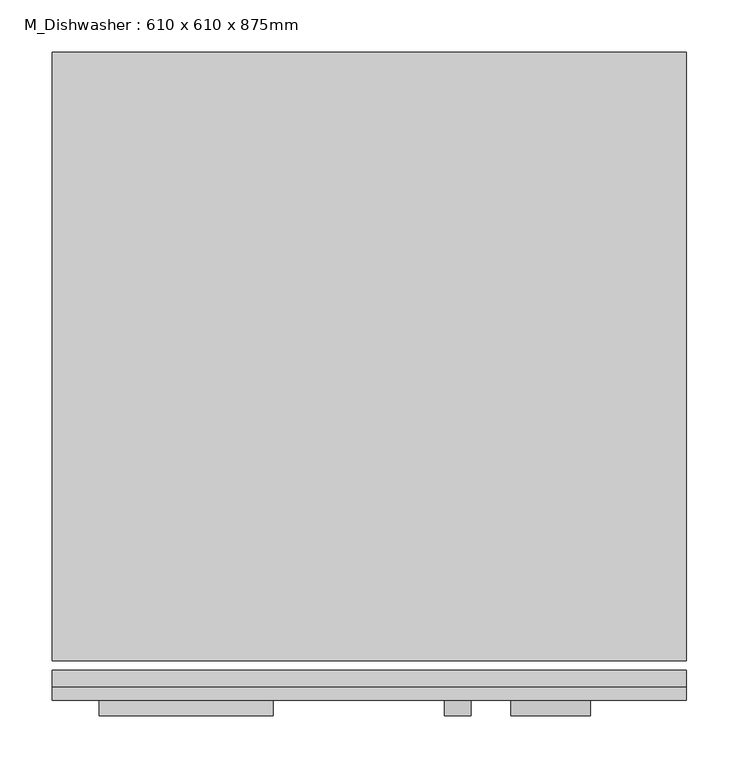
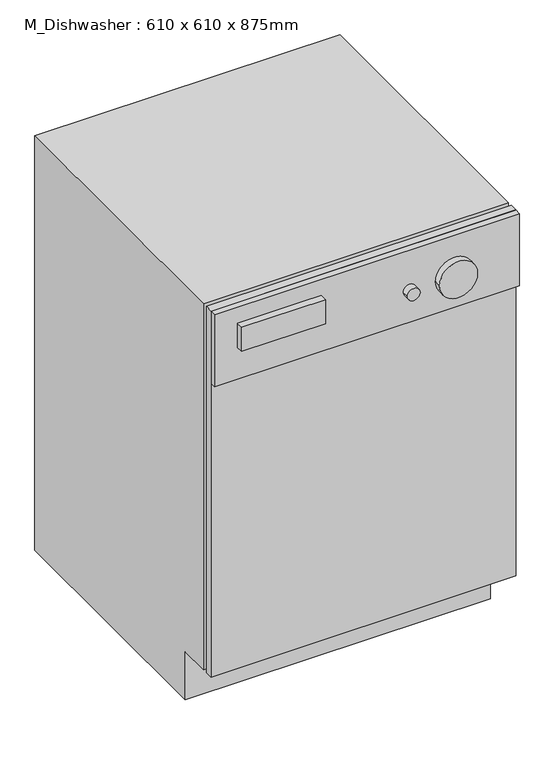
"""IFC4 building model written with IfcOpenShell, lengths in millimetres: proxy geometry, M_Dishwasher : 610 x 610 x 875mm."""

from ifc_helpers import new_model, si_unit, point, frame, frame_2d, origin, place, context, project, spatial, polyline, circle_curve, trimmed, segment, composite_curve, outline, extrude, source, transform, mapped, element, save


def m_dishwasher_610_x_610_x_875mm_54ecfc4c(model_context):
    return source(origin(), model_context, "Body", "SweptSolid", [
        extrude(outline(polyline([(687.5174685, -38.3504352), (77.5174685, -38.3504352), (77.5174685, -22.4754352), (687.5174685, -22.4754352), (687.5174685, -38.3504352)])), frame((0.0, 0.0, 101.6), z_axis=(0.0, 0.0, 1.0), x_axis=(1.0, 0.0, 0.0)), (0.0, 0.0, 1.0), 773.4),
        extrude(outline(polyline([(687.5174685, -38.3504352), (687.5174685, -51.0504352), (77.5174685, -51.0504352), (77.5174685, -38.3504352), (687.5174685, -38.3504352)])), frame((0.0, 0.0, 722.6), z_axis=(0.0, 0.0, 1.0), x_axis=(1.0, 0.0, 0.0)), (0.0, 0.0, 1.0), 152.4),
        extrude(outline(polyline([(571.6495648, 0.0), (50.5495648, 0.0), (50.5495648, 101.6), (-12.9504352, 101.6), (-12.9504352, 875.0), (571.6495648, 875.0), (571.6495648, 0.0)])), frame((77.5174685, 0.0, 0.0), z_axis=(1.0, 0.0, 0.0), x_axis=(0.0, 1.0, 0.0)), (0.0, 0.0, 1.0), 610.0),
        extrude(outline(polyline([(290.2347603, -66.0504352), (122.8347603, -66.0504352), (122.8347603, -51.0504352), (290.2347603, -51.0504352), (290.2347603, -66.0504352)])), frame((0.0, 0.0, 790.6663551), z_axis=(0.0, 0.0, 1.0), x_axis=(1.0, 0.0, 0.0)), (0.0, 0.0, 1.0), 50.8),
        extrude(outline(composite_curve([segment(trimmed(circle_curve(frame_2d((790.6663551, 467.3393328)), 12.7), [point((790.6663551, 480.0393328))], [point((790.6663551, 454.6393328))], False, "CARTESIAN"), True, "CONTINUOUS"), segment(trimmed(circle_curve(frame_2d((790.6663551, 467.3393328)), 12.7), [point((790.6663551, 454.6393328))], [point((790.6663551, 480.0393328))], False, "CARTESIAN"), True, "CONTINUOUS")], self_intersect=False)), frame((0.0, -66.0504352, 0.0), z_axis=(0.0, 1.0, 0.0), x_axis=(0.0, 0.0, 1.0)), (0.0, 0.0, 1.0), 15.0),
        extrude(outline(composite_curve([segment(trimmed(circle_curve(frame_2d((790.6663551, 556.7855874)), 38.1), [point((790.6663551, 594.8855874))], [point((790.6663551, 518.6855874))], False, "CARTESIAN"), True, "CONTINUOUS"), segment(trimmed(circle_curve(frame_2d((790.6663551, 556.7855874)), 38.1), [point((790.6663551, 518.6855874))], [point((790.6663551, 594.8855874))], False, "CARTESIAN"), True, "CONTINUOUS")], self_intersect=False)), frame((0.0, -66.0504352, 0.0), z_axis=(0.0, 1.0, 0.0), x_axis=(0.0, 0.0, 1.0)), (0.0, 0.0, 1.0), 15.0),
    ])


if __name__ == "__main__":
    model = new_model("IFC4")
    model_context = context("Model", 3, world=origin())
    ifc_project = project(units=[si_unit("LENGTHUNIT", "METRE", prefix="MILLI")], contexts=[model_context])
    site = spatial("IfcSite", under=ifc_project)
    building = spatial("IfcBuilding", under=site)
    placement = place(None, origin())
    m_dishwasher_610_x_610_x_875mm_shape = m_dishwasher_610_x_610_x_875mm_54ecfc4c(model_context)
    element("IfcBuildingElementProxy", 1, Name="M_Dishwasher : 610 x 610 x 875mm", ObjectType="M_Dishwasher : 610 x 610 x 875mm", at=placement, inside=building, context=model_context, shape_type="MappedRepresentation", body=[
        mapped(m_dishwasher_610_x_610_x_875mm_shape, transform((0.0, 0.0, 0.0), x_axis=(1.0, 0.0, 0.0), y_axis=(0.0, 1.0, 0.0), z_axis=(0.0, 0.0, 1.0))),
    ])
    save(model, "model.ifc")

# Revit data of these elements
# Type "M_Dishwasher : 610 x 610 x 875mm"
#   Label = "DW"
#   Depth = 2' - 0.01575"
#   Height = 2' - 10.44882"
#   Width = 2' - 0.01575"
#   Dishwasher Material = Steel, Paint Finish, Ivory, Glossy
#   Panel Face Material = Plastic, Opaque Black
#   Default Elevation = 0
# Element 1 (IfcBuildingElementProxy, "M_Dishwasher : 610 x 610 x 875mm")
#   Materials on its faces: "Steel, Paint Finish, Ivory, Glossy", "Plastic, Opaque Black"
# Materials
#   "Steel, Paint Finish, Ivory, Glossy": class "Metal", colour RGB 247 247 239, transparency 0, Description = "Steel, paint finish, ivory, glossy", Cost = 0
#   "Plastic, Opaque Black": class "Plastic", colour RGB 0 0 0, transparency 0.7, Description = "Plastic, generic, opaque black", Cost = 0
